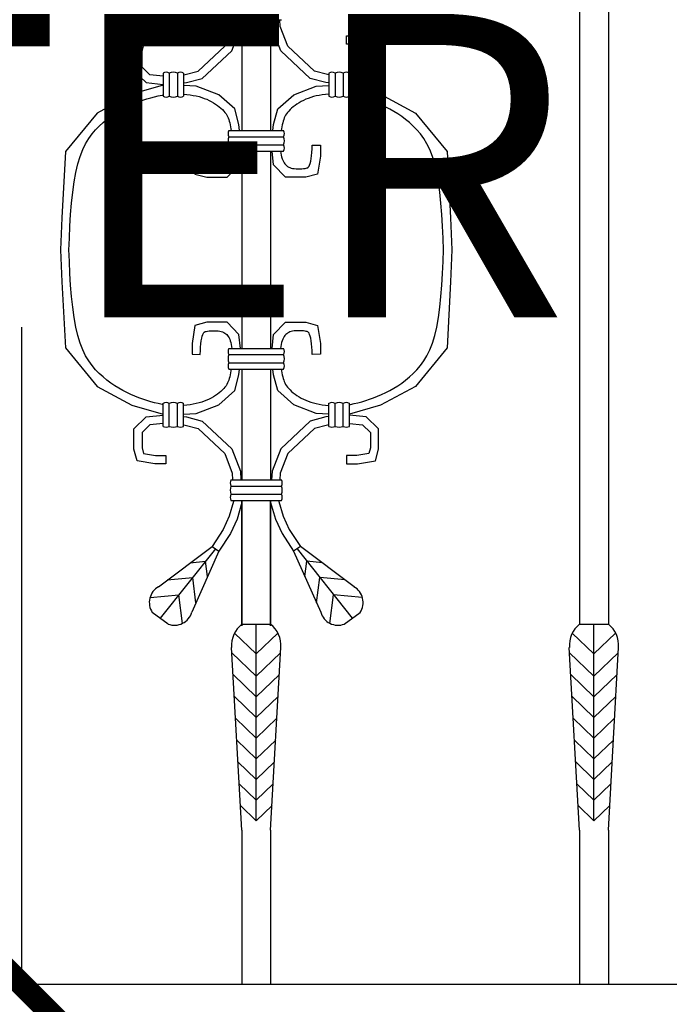
# Model space of a CAD drawing. Units: inches. Extents: x 2278 to 7495, y -71 to 1198.
# Tile 27 of 44: x 5101.34 to 5114.19, y 126.41 to 145.88. Entities that reach past the tile are written whole.
import ezdxf

# ---------------------------------------------------------------- set-up
doc = ezdxf.new("R2010")
doc.units = ezdxf.units.IN
doc.header["$MEASUREMENT"] = 0
doc.layers.add('A-ANNO-DIMS', color=2, linetype='Continuous', lineweight=18)
doc.layers.add('A-ELEV', color=7, linetype='Continuous', lineweight=25)
doc.styles.get("Standard").update_dxf_attribs({"font": 'arial.ttf'})
doc.dimstyles.get("Standard").update_dxf_attribs({"dimtxt": 6, "dimasz": 3, "dimexe": 0.18, "dimexo": 0.0625, "dimgap": 0.09, "dimtad": 0, "dimtih": 1, "dimtoh": 1, "dimdec": 0, "dimzin": 0, "dimdsep": 46, "dimlunit": 3, "dimtxsty": 'Standard', "dimblk": 'ARCHTICK', "dimcen": 0.09, "dimadec": 0, "dimazin": 0, "dimtfac": 1, "dimtdec": 0, "dimtofl": 0, "dimtmove": 0, "dimatfit": 3, "dimfxl": 1, "dimtolj": 1, "dimtzin": 0, "dimarcsym": 0})

# ---------------------------------------------------------------- blocks, each defined once
blk = doc.blocks.new('BALUSTER-ORNATE-A')
for p, q in [((3.37, 19.077), (4.37, 19.077)), ((3.396, 18.942), (3.402, 19.077)), ((3.558, 18.908), (3.565, 19.077)), ((3.585, 19.077), (3.585, 16.887)), ((4.155, 19.077), (4.155, 16.887)), ((4.182, 18.908), (4.175, 19.077)), ((4.344, 18.942), (4.338, 19.077)), ((3.247, 18.557), (3.396, 18.942)), ((3.385, 18.463), (3.558, 18.908)), ((4.355, 18.463), (4.182, 18.908)), ((4.493, 18.557), (4.344, 18.942)), ((1.513, 18.705), (1.449, 18.469)), ((1.866, 18.759), (1.513, 18.705)), ((2.084, 18.759), (1.866, 18.759)), ((2.084, 18.596), (2.084, 18.759)), ((5.656, 18.596), (5.656, 18.759)), ((5.656, 18.759), (5.874, 18.759)), ((5.874, 18.759), (6.227, 18.705)), ((6.227, 18.705), (6.291, 18.469)), ((1.612, 18.447), (1.642, 18.56)), ((1.642, 18.56), (1.879, 18.596)), ((1.879, 18.596), (2.084, 18.596)), ((2.719, 18.062), (3.247, 18.557)), ((5.021, 18.062), (4.493, 18.557)), ((5.861, 18.596), (5.656, 18.596)), ((6.098, 18.56), (5.861, 18.596)), ((6.128, 18.447), (6.098, 18.56)), ((1.449, 18.469), (1.449, 18.069)), ((1.612, 18.138), (1.612, 18.447)), ((2.801, 17.915), (3.385, 18.463)), ((4.939, 17.915), (4.355, 18.463)), ((6.128, 18.138), (6.128, 18.447)), ((6.291, 18.469), (6.291, 18.069)), ((1.767, 17.989), (1.612, 18.138)), ((5.973, 17.989), (6.128, 18.138)), ((1.449, 18.069), (1.694, 17.833)), ((2.026, 17.961), (1.767, 17.989)), ((2.026, 18.021), (2.026, 17.565)), ((2.148, 18.021), (2.148, 17.565)), ((2.311, 18.021), (2.311, 17.565)), ((2.434, 18.021), (2.434, 17.565)), ((2.434, 17.99), (2.462, 17.993)), ((2.462, 17.993), (2.719, 18.062)), ((2.492, 17.833), (2.801, 17.915)), ((5.248, 17.833), (4.939, 17.915)), ((5.278, 17.993), (5.021, 18.062)), ((5.306, 17.99), (5.278, 17.993)), ((5.306, 18.021), (5.306, 17.565)), ((5.429, 18.021), (5.429, 17.565)), ((5.592, 18.021), (5.592, 17.565)), ((5.714, 18.021), (5.714, 17.565)), ((5.714, 17.961), (5.973, 17.989)), ((6.291, 18.069), (6.046, 17.833)), ((2.026, 17.782), (1.412, 17.603)), ((1.694, 17.833), (2.026, 17.797)), ((2.434, 17.826), (2.492, 17.833)), ((2.683, 17.766), (2.434, 17.777)), ((3.128, 17.594), (2.683, 17.766)), ((4.612, 17.594), (5.057, 17.766)), ((5.057, 17.766), (5.306, 17.777)), ((5.306, 17.826), (5.248, 17.833)), ((6.046, 17.833), (5.714, 17.797)), ((5.714, 17.782), (6.328, 17.603)), ((1.412, 17.603), (0.722, 17.231)), ((1.705, 17.51), (1.782, 17.533)), ((1.782, 17.533), (1.858, 17.553)), ((1.858, 17.553), (1.933, 17.571)), ((1.933, 17.571), (2.007, 17.585)), ((2.007, 17.585), (2.026, 17.587)), ((2.434, 17.606), (2.499, 17.6)), ((2.499, 17.6), (2.563, 17.592)), ((2.563, 17.592), (2.624, 17.582)), ((2.624, 17.582), (2.683, 17.57)), ((2.683, 17.57), (2.739, 17.556)), ((2.739, 17.556), (2.792, 17.54)), ((2.792, 17.54), (2.843, 17.522)), ((2.843, 17.522), (2.891, 17.503)), ((3.446, 17.313), (3.128, 17.594)), ((4.294, 17.313), (4.612, 17.594)), ((4.897, 17.522), (4.849, 17.503)), ((4.948, 17.54), (4.897, 17.522)), ((5.001, 17.556), (4.948, 17.54)), ((5.057, 17.57), (5.001, 17.556)), ((5.116, 17.582), (5.057, 17.57)), ((5.177, 17.592), (5.116, 17.582)), ((5.241, 17.6), (5.177, 17.592)), ((5.306, 17.606), (5.241, 17.6)), ((5.733, 17.585), (5.714, 17.587)), ((5.807, 17.571), (5.733, 17.585)), ((5.882, 17.553), (5.807, 17.571)), ((5.958, 17.533), (5.882, 17.553)), ((6.035, 17.51), (5.958, 17.533)), ((6.328, 17.603), (7.018, 17.231)), ((1.23, 17.309), (1.309, 17.35)), ((1.309, 17.35), (1.389, 17.388)), ((1.389, 17.388), (1.469, 17.422)), ((1.469, 17.422), (1.549, 17.454)), ((1.549, 17.454), (1.627, 17.484)), ((1.627, 17.484), (1.705, 17.51)), ((2.891, 17.503), (2.937, 17.482)), ((2.937, 17.482), (2.981, 17.46)), ((2.981, 17.46), (3.024, 17.436)), ((3.024, 17.436), (3.064, 17.41)), ((3.064, 17.41), (3.102, 17.384)), ((3.102, 17.384), (3.138, 17.357)), ((3.138, 17.357), (3.171, 17.329)), ((3.171, 17.329), (3.201, 17.301)), ((4.569, 17.329), (4.539, 17.301)), ((4.602, 17.357), (4.569, 17.329)), ((4.638, 17.384), (4.602, 17.357)), ((4.676, 17.41), (4.638, 17.384)), ((4.716, 17.436), (4.676, 17.41)), ((4.759, 17.46), (4.716, 17.436)), ((4.803, 17.482), (4.759, 17.46)), ((4.849, 17.503), (4.803, 17.482)), ((6.113, 17.484), (6.035, 17.51)), ((6.191, 17.454), (6.113, 17.484)), ((6.271, 17.422), (6.191, 17.454)), ((6.351, 17.388), (6.271, 17.422)), ((6.431, 17.35), (6.351, 17.388)), ((6.51, 17.309), (6.431, 17.35)), ((0.722, 17.231), (0.096, 16.469)), ((0.916, 17.105), (0.993, 17.163)), ((0.993, 17.163), (1.071, 17.216)), ((1.071, 17.216), (1.15, 17.265)), ((1.15, 17.265), (1.23, 17.309)), ((3.201, 17.301), (3.228, 17.272)), ((3.228, 17.272), (3.252, 17.244)), ((3.252, 17.244), (3.272, 17.217)), ((3.272, 17.217), (3.288, 17.19)), ((3.288, 17.19), (3.303, 17.162)), ((3.303, 17.162), (3.316, 17.134)), ((3.316, 17.134), (3.327, 17.104)), ((3.528, 17.004), (3.446, 17.313)), ((4.212, 17.004), (4.294, 17.313)), ((4.424, 17.134), (4.413, 17.104)), ((4.437, 17.162), (4.424, 17.134)), ((4.452, 17.19), (4.437, 17.162)), ((4.468, 17.217), (4.452, 17.19)), ((4.489, 17.244), (4.468, 17.217)), ((4.512, 17.272), (4.489, 17.244)), ((4.539, 17.301), (4.512, 17.272)), ((6.59, 17.265), (6.51, 17.309)), ((6.669, 17.216), (6.59, 17.265)), ((6.747, 17.163), (6.669, 17.216)), ((6.824, 17.105), (6.747, 17.163)), ((7.018, 17.231), (7.644, 16.469)), ((0.692, 16.9), (0.764, 16.975)), ((0.764, 16.975), (0.839, 17.043)), ((0.839, 17.043), (0.916, 17.105)), ((3.327, 17.104), (3.337, 17.072)), ((3.337, 17.072), (3.346, 17.038)), ((3.346, 17.038), (3.354, 17.001)), ((3.354, 17.001), (3.361, 16.962)), ((3.361, 16.962), (3.368, 16.922)), ((3.542, 16.887), (3.528, 17.004)), ((4.198, 16.887), (4.212, 17.004)), ((4.379, 16.962), (4.372, 16.922)), ((4.386, 17.001), (4.379, 16.962)), ((4.394, 17.038), (4.386, 17.001)), ((4.403, 17.072), (4.394, 17.038)), ((4.413, 17.104), (4.403, 17.072)), ((6.901, 17.043), (6.824, 17.105)), ((6.976, 16.975), (6.901, 17.043)), ((7.048, 16.9), (6.976, 16.975)), ((0.557, 16.727), (0.623, 16.819)), ((0.623, 16.819), (0.692, 16.9)), ((3.329, 16.887), (4.411, 16.887)), ((3.329, 16.764), (4.411, 16.764)), ((3.368, 16.922), (3.374, 16.887)), ((4.372, 16.922), (4.366, 16.887)), ((7.117, 16.819), (7.048, 16.9)), ((7.183, 16.727), (7.117, 16.819)), ((0.438, 16.508), (0.495, 16.624)), ((0.495, 16.624), (0.557, 16.727)), ((2.764, 16.599), (2.602, 16.596)), ((2.602, 16.596), (2.602, 16.378)), ((2.766, 16.522), (2.764, 16.599)), ((3.329, 16.601), (4.411, 16.601)), ((4.974, 16.522), (4.976, 16.599)), ((4.976, 16.599), (5.138, 16.596)), ((5.138, 16.596), (5.138, 16.378)), ((7.245, 16.624), (7.183, 16.727)), ((7.302, 16.508), (7.245, 16.624)), ((0.096, 16.469), (0.025, 15.162)), ((0.34, 16.227), (0.386, 16.376)), ((0.386, 16.376), (0.438, 16.508)), ((2.602, 16.378), (2.656, 16.024)), ((2.769, 16.452), (2.766, 16.522)), ((2.775, 16.388), (2.769, 16.452)), ((2.783, 16.331), (2.775, 16.388)), ((3.329, 16.479), (4.411, 16.479)), ((3.368, 16.364), (3.357, 16.329)), ((3.376, 16.401), (3.368, 16.364)), ((3.383, 16.441), (3.376, 16.401)), ((3.388, 16.479), (3.383, 16.441)), ((3.528, 16.206), (3.557, 16.479)), ((3.585, 16.479), (3.585, 12.578)), ((4.155, 16.479), (4.155, 12.578)), ((4.212, 16.206), (4.183, 16.479)), ((4.352, 16.479), (4.357, 16.441)), ((4.357, 16.441), (4.364, 16.401)), ((4.364, 16.401), (4.372, 16.364)), ((4.372, 16.364), (4.383, 16.329)), ((4.957, 16.331), (4.965, 16.388)), ((4.965, 16.388), (4.971, 16.452)), ((4.971, 16.452), (4.974, 16.522)), ((5.138, 16.378), (5.084, 16.024)), ((7.354, 16.376), (7.302, 16.508)), ((7.4, 16.227), (7.354, 16.376)), ((7.644, 16.469), (7.715, 15.162)), ((0.3, 16.057), (0.34, 16.227)), ((2.792, 16.28), (2.783, 16.331)), ((2.803, 16.237), (2.792, 16.28)), ((2.815, 16.203), (2.803, 16.237)), ((2.825, 16.18), (2.815, 16.203)), ((2.834, 16.166), (2.825, 16.18)), ((2.84, 16.159), (2.834, 16.166)), ((2.846, 16.154), (2.84, 16.159)), ((3.228, 16.164), (3.205, 16.154)), ((3.249, 16.176), (3.228, 16.164)), ((3.268, 16.19), (3.249, 16.176)), ((3.286, 16.207), (3.268, 16.19)), ((3.303, 16.225), (3.286, 16.207)), ((3.292, 15.961), (3.528, 16.206)), ((3.318, 16.247), (3.303, 16.225)), ((3.333, 16.271), (3.318, 16.247)), ((3.346, 16.299), (3.333, 16.271)), ((3.357, 16.329), (3.346, 16.299)), ((4.448, 15.961), (4.212, 16.206)), ((4.383, 16.329), (4.394, 16.299)), ((4.394, 16.299), (4.407, 16.271)), ((4.407, 16.271), (4.422, 16.247)), ((4.422, 16.247), (4.437, 16.225)), ((4.437, 16.225), (4.454, 16.207)), ((4.454, 16.207), (4.472, 16.19)), ((4.472, 16.19), (4.491, 16.176)), ((4.491, 16.176), (4.512, 16.164)), ((4.512, 16.164), (4.535, 16.154)), ((4.895, 16.154), (4.9, 16.159)), ((4.9, 16.159), (4.906, 16.166)), ((4.906, 16.166), (4.915, 16.18)), ((4.915, 16.18), (4.925, 16.203)), ((4.925, 16.203), (4.937, 16.237)), ((4.937, 16.237), (4.948, 16.28)), ((4.948, 16.28), (4.957, 16.331)), ((7.44, 16.057), (7.4, 16.227)), ((0.267, 15.87), (0.3, 16.057)), ((2.656, 16.024), (2.892, 15.961)), ((2.852, 16.151), (2.846, 16.154)), ((2.863, 16.146), (2.852, 16.151)), ((2.88, 16.142), (2.863, 16.146)), ((2.905, 16.137), (2.88, 16.142)), ((2.936, 16.134), (2.905, 16.137)), ((2.971, 16.131), (2.936, 16.134)), ((3.008, 16.129), (2.971, 16.131)), ((3.045, 16.129), (3.008, 16.129)), ((3.081, 16.13), (3.045, 16.129)), ((3.117, 16.133), (3.081, 16.13)), ((3.15, 16.138), (3.117, 16.133)), ((3.179, 16.145), (3.15, 16.138)), ((3.205, 16.154), (3.179, 16.145)), ((4.535, 16.154), (4.561, 16.145)), ((4.561, 16.145), (4.59, 16.138)), ((4.59, 16.138), (4.623, 16.133)), ((4.623, 16.133), (4.659, 16.13)), ((4.659, 16.13), (4.695, 16.129)), ((4.695, 16.129), (4.732, 16.129)), ((4.732, 16.129), (4.769, 16.131)), ((4.769, 16.131), (4.804, 16.134)), ((4.804, 16.134), (4.835, 16.137)), ((4.835, 16.137), (4.86, 16.142)), ((5.084, 16.024), (4.848, 15.961)), ((4.86, 16.142), (4.877, 16.146)), ((4.877, 16.146), (4.888, 16.151)), ((4.888, 16.151), (4.895, 16.154)), ((7.473, 15.87), (7.44, 16.057)), ((0.239, 15.667), (0.267, 15.87)), ((2.892, 15.961), (3.292, 15.961)), ((4.848, 15.961), (4.448, 15.961)), ((7.501, 15.667), (7.473, 15.87)), ((0.217, 15.452), (0.239, 15.667)), ((7.523, 15.452), (7.501, 15.667)), ((0.199, 15.227), (0.217, 15.452)), ((7.541, 15.227), (7.523, 15.452)), ((0.185, 14.995), (0.199, 15.227)), ((7.555, 14.995), (7.541, 15.227)), ((0.025, 15.162), (0, 14.529)), ((0.173, 14.759), (0.185, 14.995)), ((7.567, 14.759), (7.555, 14.995)), ((7.715, 15.162), (7.74, 14.529)), ((0.163, 14.522), (0.173, 14.759)), ((7.577, 14.522), (7.567, 14.759)), ((0, 14.529), (0.025, 13.895)), ((0.173, 14.298), (0.163, 14.536)), ((7.567, 14.298), (7.577, 14.536)), ((7.74, 14.529), (7.715, 13.895)), ((0.185, 14.062), (0.173, 14.298)), ((7.555, 14.062), (7.567, 14.298)), ((0.199, 13.831), (0.185, 14.062)), ((7.541, 13.831), (7.555, 14.062)), ((0.025, 13.895), (0.096, 12.589)), ((0.217, 13.606), (0.199, 13.831)), ((7.523, 13.606), (7.541, 13.831)), ((7.715, 13.895), (7.644, 12.589)), ((0.239, 13.391), (0.217, 13.606)), ((7.501, 13.391), (7.523, 13.606)), ((0.267, 13.188), (0.239, 13.391)), ((7.473, 13.188), (7.501, 13.391)), ((0.3, 13), (0.267, 13.188)), ((2.892, 13.097), (2.656, 13.033)), ((3.292, 13.097), (2.892, 13.097)), ((3.528, 12.852), (3.292, 13.097)), ((4.212, 12.852), (4.448, 13.097)), ((4.448, 13.097), (4.848, 13.097)), ((4.848, 13.097), (5.084, 13.033)), ((7.44, 13), (7.473, 13.188)), ((0.34, 12.831), (0.3, 13)), ((2.656, 13.033), (2.602, 12.679)), ((2.803, 12.82), (2.815, 12.854)), ((2.815, 12.854), (2.825, 12.878)), ((2.825, 12.878), (2.834, 12.892)), ((2.834, 12.892), (2.84, 12.899)), ((2.84, 12.899), (2.846, 12.903)), ((2.846, 12.903), (2.852, 12.907)), ((2.852, 12.907), (2.863, 12.911)), ((2.863, 12.911), (2.88, 12.916)), ((2.88, 12.916), (2.905, 12.92)), ((2.905, 12.92), (2.936, 12.924)), ((2.936, 12.924), (2.971, 12.927)), ((2.971, 12.927), (3.008, 12.929)), ((3.008, 12.929), (3.045, 12.929)), ((3.045, 12.929), (3.081, 12.928)), ((3.081, 12.928), (3.117, 12.924)), ((3.117, 12.924), (3.15, 12.919)), ((3.15, 12.919), (3.179, 12.912)), ((3.179, 12.912), (3.205, 12.904)), ((3.205, 12.904), (3.228, 12.893)), ((3.228, 12.893), (3.249, 12.881)), ((3.249, 12.881), (3.268, 12.867)), ((3.268, 12.867), (3.286, 12.851)), ((3.286, 12.851), (3.303, 12.832)), ((3.557, 12.578), (3.528, 12.852)), ((4.183, 12.578), (4.212, 12.852)), ((4.454, 12.851), (4.437, 12.832)), ((4.472, 12.867), (4.454, 12.851)), ((4.491, 12.881), (4.472, 12.867)), ((4.512, 12.893), (4.491, 12.881)), ((4.535, 12.904), (4.512, 12.893)), ((4.561, 12.912), (4.535, 12.904)), ((4.59, 12.919), (4.561, 12.912)), ((4.623, 12.924), (4.59, 12.919)), ((4.659, 12.928), (4.623, 12.924)), ((4.695, 12.929), (4.659, 12.928)), ((4.732, 12.929), (4.695, 12.929)), ((4.769, 12.927), (4.732, 12.929)), ((4.804, 12.924), (4.769, 12.927)), ((4.835, 12.92), (4.804, 12.924)), ((4.86, 12.916), (4.835, 12.92)), ((4.877, 12.911), (4.86, 12.916)), ((4.888, 12.907), (4.877, 12.911)), ((4.895, 12.903), (4.888, 12.907)), ((4.9, 12.899), (4.895, 12.903)), ((4.906, 12.892), (4.9, 12.899)), ((4.915, 12.878), (4.906, 12.892)), ((4.925, 12.854), (4.915, 12.878)), ((4.937, 12.82), (4.925, 12.854)), ((5.084, 13.033), (5.138, 12.679)), ((7.4, 12.831), (7.44, 13)), ((0.386, 12.681), (0.34, 12.831)), ((0.438, 12.549), (0.386, 12.681)), ((2.602, 12.679), (2.602, 12.462)), ((2.769, 12.605), (2.775, 12.669)), ((2.775, 12.669), (2.783, 12.727)), ((2.783, 12.727), (2.792, 12.778)), ((2.792, 12.778), (2.803, 12.82)), ((3.303, 12.832), (3.318, 12.811)), ((3.318, 12.811), (3.333, 12.786)), ((3.333, 12.786), (3.346, 12.759)), ((3.346, 12.759), (3.357, 12.728)), ((3.357, 12.728), (3.368, 12.694)), ((3.368, 12.694), (3.376, 12.656)), ((3.376, 12.656), (3.383, 12.616)), ((4.364, 12.656), (4.357, 12.616)), ((4.372, 12.694), (4.364, 12.656)), ((4.383, 12.728), (4.372, 12.694)), ((4.394, 12.759), (4.383, 12.728)), ((4.407, 12.786), (4.394, 12.759)), ((4.422, 12.811), (4.407, 12.786)), ((4.437, 12.832), (4.422, 12.811)), ((4.948, 12.778), (4.937, 12.82)), ((4.957, 12.727), (4.948, 12.778)), ((4.965, 12.669), (4.957, 12.727)), ((4.971, 12.605), (4.965, 12.669)), ((5.138, 12.679), (5.138, 12.462)), ((7.302, 12.549), (7.354, 12.681)), ((7.354, 12.681), (7.4, 12.831)), ((0.096, 12.589), (0.722, 11.827)), ((0.495, 12.433), (0.438, 12.549)), ((2.602, 12.462), (2.764, 12.459)), ((2.764, 12.459), (2.766, 12.536)), ((2.766, 12.536), (2.769, 12.605)), ((3.329, 12.578), (4.411, 12.578)), ((3.383, 12.616), (3.388, 12.578)), ((4.357, 12.616), (4.352, 12.578)), ((4.974, 12.536), (4.971, 12.605)), ((4.976, 12.459), (4.974, 12.536)), ((5.138, 12.462), (4.976, 12.459)), ((7.644, 12.589), (7.018, 11.827)), ((7.245, 12.433), (7.302, 12.549)), ((0.557, 12.33), (0.495, 12.433)), ((0.623, 12.239), (0.557, 12.33)), ((3.329, 12.456), (4.411, 12.456)), ((3.329, 12.293), (4.411, 12.293)), ((7.117, 12.239), (7.183, 12.33)), ((7.183, 12.33), (7.245, 12.433)), ((0.692, 12.157), (0.623, 12.239)), ((0.764, 12.083), (0.692, 12.157)), ((0.839, 12.015), (0.764, 12.083)), ((3.329, 12.171), (4.411, 12.171)), ((3.361, 12.095), (3.354, 12.056)), ((3.368, 12.136), (3.361, 12.095)), ((3.374, 12.171), (3.368, 12.136)), ((3.528, 12.053), (3.542, 12.171)), ((3.585, 12.171), (3.585, 9.98)), ((4.155, 12.171), (4.155, 9.98)), ((4.212, 12.053), (4.198, 12.171)), ((4.366, 12.171), (4.372, 12.136)), ((4.372, 12.136), (4.379, 12.095)), ((4.379, 12.095), (4.386, 12.056)), ((6.901, 12.015), (6.976, 12.083)), ((6.976, 12.083), (7.048, 12.157)), ((7.048, 12.157), (7.117, 12.239)), ((0.916, 11.952), (0.839, 12.015)), ((0.993, 11.894), (0.916, 11.952)), ((1.071, 11.841), (0.993, 11.894)), ((3.303, 11.895), (3.288, 11.868)), ((3.316, 11.924), (3.303, 11.895)), ((3.327, 11.954), (3.316, 11.924)), ((3.337, 11.986), (3.327, 11.954)), ((3.346, 12.02), (3.337, 11.986)), ((3.354, 12.056), (3.346, 12.02)), ((3.446, 11.745), (3.528, 12.053)), ((4.294, 11.745), (4.212, 12.053)), ((4.386, 12.056), (4.394, 12.02)), ((4.394, 12.02), (4.403, 11.986)), ((4.403, 11.986), (4.413, 11.954)), ((4.413, 11.954), (4.424, 11.924)), ((4.424, 11.924), (4.437, 11.895)), ((4.437, 11.895), (4.452, 11.868)), ((6.669, 11.841), (6.747, 11.894)), ((6.747, 11.894), (6.824, 11.952)), ((6.824, 11.952), (6.901, 12.015)), ((0.722, 11.827), (1.412, 11.455)), ((1.15, 11.793), (1.071, 11.841)), ((1.23, 11.748), (1.15, 11.793)), ((1.309, 11.708), (1.23, 11.748)), ((1.389, 11.67), (1.309, 11.708)), ((3.138, 11.701), (3.102, 11.673)), ((3.128, 11.464), (3.446, 11.745)), ((3.171, 11.729), (3.138, 11.701)), ((3.201, 11.757), (3.171, 11.729)), ((3.228, 11.785), (3.201, 11.757)), ((3.252, 11.813), (3.228, 11.785)), ((3.272, 11.841), (3.252, 11.813)), ((3.288, 11.868), (3.272, 11.841)), ((4.612, 11.464), (4.294, 11.745)), ((4.452, 11.868), (4.468, 11.841)), ((4.468, 11.841), (4.489, 11.813)), ((4.489, 11.813), (4.512, 11.785)), ((4.512, 11.785), (4.539, 11.757)), ((4.539, 11.757), (4.569, 11.729)), ((4.569, 11.729), (4.602, 11.701)), ((4.602, 11.701), (4.638, 11.673)), ((7.018, 11.827), (6.328, 11.455)), ((6.351, 11.67), (6.431, 11.708)), ((6.431, 11.708), (6.51, 11.748)), ((6.51, 11.748), (6.59, 11.793)), ((6.59, 11.793), (6.669, 11.841)), ((1.469, 11.635), (1.389, 11.67)), ((1.549, 11.603), (1.469, 11.635)), ((1.627, 11.574), (1.549, 11.603)), ((1.705, 11.548), (1.627, 11.574)), ((1.782, 11.524), (1.705, 11.548)), ((1.858, 11.504), (1.782, 11.524)), ((1.933, 11.487), (1.858, 11.504)), ((2.007, 11.473), (1.933, 11.487)), ((2.026, 11.037), (2.026, 11.493)), ((2.148, 11.037), (2.148, 11.493)), ((2.311, 11.037), (2.311, 11.493)), ((2.434, 11.037), (2.434, 11.493)), ((2.683, 11.488), (2.624, 11.476)), ((2.739, 11.502), (2.683, 11.488)), ((2.792, 11.518), (2.739, 11.502)), ((2.843, 11.535), (2.792, 11.518)), ((2.891, 11.555), (2.843, 11.535)), ((2.937, 11.576), (2.891, 11.555)), ((2.981, 11.598), (2.937, 11.576)), ((3.024, 11.622), (2.981, 11.598)), ((3.064, 11.647), (3.024, 11.622)), ((3.102, 11.673), (3.064, 11.647)), ((4.638, 11.673), (4.676, 11.647)), ((4.676, 11.647), (4.716, 11.622)), ((4.716, 11.622), (4.759, 11.598)), ((4.759, 11.598), (4.803, 11.576)), ((4.803, 11.576), (4.849, 11.555)), ((4.849, 11.555), (4.897, 11.535)), ((4.897, 11.535), (4.948, 11.518)), ((4.948, 11.518), (5.001, 11.502)), ((5.001, 11.502), (5.057, 11.488)), ((5.057, 11.488), (5.116, 11.476)), ((5.306, 11.037), (5.306, 11.493)), ((5.429, 11.037), (5.429, 11.493)), ((5.592, 11.037), (5.592, 11.493)), ((5.714, 11.037), (5.714, 11.493)), ((5.733, 11.473), (5.807, 11.487)), ((5.807, 11.487), (5.882, 11.504)), ((5.882, 11.504), (5.958, 11.524)), ((5.958, 11.524), (6.035, 11.548)), ((6.035, 11.548), (6.113, 11.574)), ((6.113, 11.574), (6.191, 11.603)), ((6.191, 11.603), (6.271, 11.635)), ((6.271, 11.635), (6.351, 11.67)), ((1.412, 11.455), (2.026, 11.276)), ((2.026, 11.47), (2.007, 11.473)), ((2.499, 11.457), (2.434, 11.451)), ((2.434, 11.28), (2.683, 11.291)), ((2.563, 11.465), (2.499, 11.457)), ((2.624, 11.476), (2.563, 11.465)), ((2.683, 11.291), (3.128, 11.464)), ((5.057, 11.291), (4.612, 11.464)), ((5.306, 11.28), (5.057, 11.291)), ((5.116, 11.476), (5.177, 11.465)), ((5.177, 11.465), (5.241, 11.457)), ((5.241, 11.457), (5.306, 11.451)), ((5.714, 11.47), (5.733, 11.473)), ((6.328, 11.455), (5.714, 11.276)), ((1.449, 10.988), (1.694, 11.225)), ((1.694, 11.225), (2.026, 11.261)), ((2.026, 11.097), (1.767, 11.069)), ((2.434, 11.232), (2.492, 11.225)), ((2.492, 11.225), (2.801, 11.143)), ((2.801, 11.143), (3.385, 10.594)), ((4.939, 11.143), (4.355, 10.594)), ((5.248, 11.225), (4.939, 11.143)), ((5.306, 11.232), (5.248, 11.225)), ((6.046, 11.225), (5.714, 11.261)), ((5.714, 11.097), (5.973, 11.069)), ((6.291, 10.988), (6.046, 11.225)), ((1.449, 10.589), (1.449, 10.988)), ((1.767, 11.069), (1.612, 10.919)), ((1.612, 10.919), (1.612, 10.611)), ((2.434, 11.067), (2.462, 11.064)), ((2.462, 11.064), (2.719, 10.996)), ((2.719, 10.996), (3.247, 10.501)), ((5.021, 10.996), (4.493, 10.501)), ((5.278, 11.064), (5.021, 10.996)), ((5.306, 11.067), (5.278, 11.064)), ((5.973, 11.069), (6.128, 10.919)), ((6.128, 10.919), (6.128, 10.611)), ((6.291, 10.589), (6.291, 10.988)), ((1.513, 10.353), (1.449, 10.589)), ((1.612, 10.611), (1.642, 10.498)), ((3.385, 10.594), (3.558, 10.149)), ((4.355, 10.594), (4.182, 10.149)), ((6.128, 10.611), (6.098, 10.498)), ((6.227, 10.353), (6.291, 10.589)), ((1.866, 10.298), (1.513, 10.353)), ((1.642, 10.498), (1.879, 10.461)), ((1.879, 10.461), (2.084, 10.461)), ((2.084, 10.461), (2.084, 10.298)), ((3.247, 10.501), (3.396, 10.115)), ((4.493, 10.501), (4.344, 10.115)), ((5.861, 10.461), (5.656, 10.461)), ((5.656, 10.461), (5.656, 10.298)), ((6.098, 10.498), (5.861, 10.461)), ((5.874, 10.298), (6.227, 10.353)), ((2.084, 10.298), (1.866, 10.298)), ((3.558, 10.149), (3.565, 9.98)), ((4.182, 10.149), (4.175, 9.98)), ((5.656, 10.298), (5.874, 10.298)), ((3.37, 9.98), (4.37, 9.98)), ((3.396, 10.115), (3.402, 9.98)), ((4.344, 10.115), (4.338, 9.98)), ((3.37, 9.858), (4.37, 9.858)), ((3.421, 9.552), (3.337, 9.262)), ((3.37, 9.695), (4.37, 9.695)), ((3.37, 9.573), (4.37, 9.573)), ((3.42, 9.573), (3.421, 9.552)), ((3.583, 9.573), (3.585, 9.532)), ((3.585, 9.573), (3.585, 7.095)), ((3.585, 7.095), (3.585, 9.573)), ((4.155, 9.573), (4.155, 7.095)), ((4.155, 7.095), (4.155, 9.573)), ((4.157, 9.573), (4.155, 9.532)), ((4.32, 9.573), (4.319, 9.552)), ((4.319, 9.552), (4.403, 9.262)), ((3.585, 9.532), (3.49, 9.205)), ((4.155, 9.532), (4.25, 9.205)), ((3.337, 9.262), (3.217, 9.001)), ((3.49, 9.205), (3.36, 8.922)), ((4.25, 9.205), (4.38, 8.922)), ((4.403, 9.262), (4.523, 9.001)), ((3.217, 9.001), (2.995, 8.66)), ((4.523, 9.001), (4.745, 8.66)), ((3.36, 8.922), (3.131, 8.571)), ((4.38, 8.922), (4.609, 8.571)), ((1.936, 7.866), (2.995, 8.66)), ((3.063, 8.615), (1.97, 7.244)), ((3.131, 8.571), (2.594, 7.362)), ((2.995, 8.66), (3.131, 8.571)), ((4.745, 8.66), (4.609, 8.571)), ((4.609, 8.571), (5.146, 7.362)), ((4.677, 8.615), (5.77, 7.244)), ((5.804, 7.866), (4.745, 8.66)), ((2.562, 8.34), (2.868, 8.37)), ((2.907, 8.066), (2.868, 8.37)), ((4.833, 8.066), (4.872, 8.37)), ((5.178, 8.34), (4.872, 8.37)), ((2.111, 8.002), (2.613, 8.051)), ((2.678, 7.551), (2.613, 8.051)), ((5.062, 7.551), (5.127, 8.051)), ((5.629, 8.002), (5.127, 8.051)), ((1.774, 7.651), (2.339, 7.706)), ((2.412, 7.143), (2.339, 7.706)), ((5.328, 7.143), (5.401, 7.706)), ((5.966, 7.651), (5.401, 7.706)), ((2.128, 7.128), (1.813, 7.359)), ((5.612, 7.128), (5.927, 7.359)), ((3.585, 7.128), (4.155, 7.128)), ((3.87, 3.24), (3.87, 7.128)), ((3.442, 6.952), (3.87, 6.538)), ((4.299, 6.952), (3.87, 6.538)), ((3.585, 3.055), (3.383, 6.664)), ((4.155, 3.055), (4.357, 6.664)), ((3.388, 6.562), (3.87, 6.097)), ((4.352, 6.562), (3.87, 6.097)), ((3.413, 6.131), (3.87, 5.689)), ((4.327, 6.131), (3.87, 5.689)), ((3.437, 5.699), (3.87, 5.28)), ((4.303, 5.699), (3.87, 5.28)), ((3.461, 5.268), (3.87, 4.872)), ((4.279, 5.268), (3.87, 4.872)), ((3.485, 4.836), (3.87, 4.464)), ((4.255, 4.836), (3.87, 4.464)), ((3.509, 4.405), (3.87, 4.056)), ((4.231, 4.405), (3.87, 4.056)), ((3.533, 3.973), (3.87, 3.648)), ((4.207, 3.973), (3.87, 3.648)), ((3.558, 3.542), (3.87, 3.24)), ((4.182, 3.542), (3.87, 3.24)), ((3.585, 3.055), (3.585, 0)), ((4.155, 3.055), (4.155, 0))]:
    blk.add_line(p, q)
for centre, radius, start, end in [((2.087, 17.916), 0.121, 59.7768, 120.2232), ((2.23, 17.828), 0.209, 67.1017, 112.8983), ((2.373, 17.916), 0.121, 59.7768, 120.2232), ((5.368, 17.916), 0.121, 59.7768, 120.2232), ((5.51, 17.828), 0.209, 67.1017, 112.8983), ((5.653, 17.916), 0.121, 59.7768, 120.2232), ((2.087, 17.67), 0.121, 239.7768, 300.2232), ((2.23, 17.758), 0.209, 247.1017, 292.8983), ((2.373, 17.67), 0.121, 239.7768, 300.2232), ((5.368, 17.67), 0.121, 239.7768, 300.2232), ((5.51, 17.758), 0.209, 247.1017, 292.8983), ((5.653, 17.67), 0.121, 239.7768, 300.2232), ((3.434, 16.825), 0.121, 149.7768, 210.2232), ((3.522, 16.683), 0.209, 157.1017, 202.8983), ((4.306, 16.825), 0.121, 329.7768, 30.2232), ((4.218, 16.683), 0.209, 337.1017, 22.8983), ((3.434, 16.54), 0.121, 149.7768, 210.2232), ((4.306, 16.54), 0.121, 329.7768, 30.2232), ((3.434, 12.517), 0.121, 149.7768, 210.2232), ((4.306, 12.517), 0.121, 329.7768, 30.2232), ((3.522, 12.375), 0.209, 157.1017, 202.8983), ((3.434, 12.232), 0.121, 149.7768, 210.2232), ((4.218, 12.375), 0.209, 337.1017, 22.8983), ((4.306, 12.232), 0.121, 329.7768, 30.2232), ((2.087, 11.388), 0.121, 59.7768, 120.2232), ((2.23, 11.3), 0.209, 67.1017, 112.8983), ((2.373, 11.388), 0.121, 59.7768, 120.2232), ((5.368, 11.388), 0.121, 59.7768, 120.2232), ((5.51, 11.3), 0.209, 67.1017, 112.8983), ((5.653, 11.388), 0.121, 59.7768, 120.2232), ((2.087, 11.142), 0.121, 239.7768, 300.2232), ((2.23, 11.23), 0.209, 247.1017, 292.8983), ((2.373, 11.142), 0.121, 239.7768, 300.2232), ((5.368, 11.142), 0.121, 239.7768, 300.2232), ((5.51, 11.23), 0.209, 247.1017, 292.8983), ((5.653, 11.142), 0.121, 239.7768, 300.2232), ((3.475, 9.919), 0.121, 149.7768, 210.2232), ((4.265, 9.919), 0.121, 329.7768, 30.2232), ((3.563, 9.776), 0.209, 157.1017, 202.8983), ((4.177, 9.776), 0.209, 337.1017, 22.8983), ((3.475, 9.634), 0.121, 149.7768, 210.2232), ((4.265, 9.634), 0.121, 329.7768, 30.2232), ((2.111, 7.555), 0.356, 119.3212, 213.425), ((5.629, 7.555), 0.356, 326.575, 60.6788), ((2.253, 7.462), 0.356, 249.4937, 343.5975), ((5.487, 7.462), 0.356, 196.4025, 290.5063), ((3.929, 6.703), 0.547, 128.9283, 183.9822), ((3.811, 6.703), 0.547, 356.0178, 51.0717)]:
    blk.add_arc(centre, radius, start, end)
blk = doc.blocks.new('RAIL-BAR-C')
for p, q in [((0.203, 21.929), (0.203, 7.128)), ((0.773, 21.929), (0.773, 7.128)), ((0.203, 7.128), (0.773, 7.128)), ((0.488, 3.24), (0.488, 7.128)), ((0.059, 6.952), (0.488, 6.538)), ((0.916, 6.952), (0.488, 6.538)), ((0.203, 3.055), (0, 6.664)), ((0.773, 3.055), (0.975, 6.664)), ((0.006, 6.562), (0.488, 6.097)), ((0.969, 6.562), (0.488, 6.097)), ((0.03, 6.131), (0.488, 5.689)), ((0.945, 6.131), (0.488, 5.689)), ((0.054, 5.699), (0.488, 5.28)), ((0.921, 5.699), (0.488, 5.28)), ((0.079, 5.268), (0.488, 4.872)), ((0.897, 5.268), (0.488, 4.872)), ((0.103, 4.836), (0.488, 4.464)), ((0.873, 4.836), (0.488, 4.464)), ((0.127, 4.405), (0.488, 4.056)), ((0.848, 4.405), (0.488, 4.056)), ((0.151, 3.973), (0.488, 3.648)), ((0.824, 3.973), (0.488, 3.648)), ((0.175, 3.542), (0.488, 3.24)), ((0.8, 3.542), (0.488, 3.24)), ((0.203, 3.055), (0.203, 0)), ((0.773, 3.055), (0.773, 0))]:
    blk.add_line(p, q)
for centre, start, end in [((0.547, 6.703), 128.9283, 183.9822), ((0.429, 6.703), 356.0178, 51.0717)]:
    blk.add_arc(centre, 0.547, start, end)
blk = doc.blocks.new('_ArchTick')
at = {"color": 0, "linetype": 'ByBlock', "const_width": 0.15}
blk.add_lwpolyline([(-0.5, -0.5), (0.5, 0.5)], dxfattribs=at)
blk = doc.blocks.new('*D59')
at = {"layer": 'A-ANNO-DIMS', "color": 0, "lineweight": -2, "transparency": 16777216}
for p, q in [((5096.589, 159.183), (5101.564, 159.183)), ((5101.384, 159.183), (5101.384, 146.185)), ((5101.384, 126.799), (5101.384, 139.796)), ((5096.589, 126.799), (5101.564, 126.799))]:
    blk.add_line(p, q, dxfattribs=at)
at = {"layer": 'Defpoints', "color": 0, "transparency": 16777216}
for p in [(5096.527, 159.183), (5101.384, 159.183), (5096.527, 126.799)]:
    blk.add_point(p, dxfattribs=at)
at = {"layer": 'A-ANNO-DIMS', "color": 0, "lineweight": -2, "transparency": 16777216, "xscale": 3, "yscale": 3, "zscale": 3}
for p, rotation in [((5101.384, 159.183), 90), ((5101.384, 126.799), 270)]:
    blk.add_blockref('_ArchTick', p, dxfattribs=dict(at, rotation=rotation))
at = {"layer": 'A-ANNO-DIMS', "color": 0, "transparency": 16777216, "insert": (5101.384, 142.991), "char_height": 6, "attachment_point": 5}
blk.add_mtext('\\A1;ORNATE BALUSTER 2\'-8 1/2" TYP.', dxfattribs=at)
blk = doc.blocks.new('*D60')
at = {"layer": 'A-ANNO-DIMS', "color": 0, "lineweight": -2, "transparency": 16777216}
for p, q in [((5088.787, 126.736), (5088.787, 121.761)), ((5096.527, 126.736), (5096.527, 121.761)), ((5088.787, 121.941), (5096.527, 121.941)), ((5096.527, 121.941), (5099.527, 121.941))]:
    blk.add_line(p, q, dxfattribs=at)
at = {"layer": 'Defpoints', "color": 0, "transparency": 16777216}
for p in [(5088.787, 126.799), (5096.527, 126.799), (5096.527, 121.941)]:
    blk.add_point(p, dxfattribs=at)
at = {"layer": 'A-ANNO-DIMS', "color": 0, "lineweight": -2, "transparency": 16777216, "xscale": 3, "yscale": 3, "zscale": 3, "rotation": 180}
blk.add_blockref('_ArchTick', (5088.787, 121.941), dxfattribs=at)
at = {"layer": 'A-ANNO-DIMS', "color": 0, "lineweight": -2, "transparency": 16777216, "xscale": 3, "yscale": 3, "zscale": 3}
blk.add_blockref('_ArchTick', (5096.527, 121.941), dxfattribs=at)
at = {"layer": 'A-ANNO-DIMS', "color": 0, "transparency": 16777216, "insert": (5124.894, 121.941), "char_height": 6, "attachment_point": 5}
blk.add_mtext('\\A1;0\'-7 1/2" TYP.', dxfattribs=at)
blk = doc.blocks.new('*D123')
at = {"layer": 'A-ANNO-DIMS', "color": 0, "lineweight": -2, "transparency": 16777216}
for p, q in [((4736.95, 340.157), (4736.95, -23.427)), ((5145.676, -1.81), (5145.676, -23.427)), ((4736.95, -23.247), (4923.929, -23.247)), ((5145.676, -23.247), (4958.697, -23.247))]:
    blk.add_line(p, q, dxfattribs=at)
at = {"layer": 'Defpoints', "color": 0, "transparency": 16777216}
for p in [(4736.95, 340.219), (5145.676, -1.747), (5145.676, -23.247)]:
    blk.add_point(p, dxfattribs=at)
at = {"layer": 'A-ANNO-DIMS', "color": 0, "lineweight": -2, "transparency": 16777216, "xscale": 3, "yscale": 3, "zscale": 3, "rotation": 180}
blk.add_blockref('_ArchTick', (4736.95, -23.247), dxfattribs=at)
at = {"layer": 'A-ANNO-DIMS', "color": 0, "lineweight": -2, "transparency": 16777216, "xscale": 3, "yscale": 3, "zscale": 3}
blk.add_blockref('_ArchTick', (5145.676, -23.247), dxfattribs=at)
at = {"layer": 'A-ANNO-DIMS', "color": 0, "transparency": 16777216, "insert": (4941.313, -23.247), "char_height": 6, "attachment_point": 5}
blk.add_mtext('\\A1;34\'-0 1/2"', dxfattribs=at)
blk = doc.blocks.new('*D131')
at = {"layer": 'A-ANNO-DIMS', "color": 0, "lineweight": -2, "transparency": 16777216}
for p, q in [((5096.176, 99.315), (5096.176, 361.899)), ((5145.676, 118.315), (5145.676, 361.899)), ((5096.176, 361.719), (5105.75, 361.719)), ((5145.676, 361.719), (5136.102, 361.719))]:
    blk.add_line(p, q, dxfattribs=at)
at = {"layer": 'Defpoints', "color": 0, "transparency": 16777216}
for p in [(5145.676, 361.719), (5145.676, 118.253), (5096.176, 99.253)]:
    blk.add_point(p, dxfattribs=at)
at = {"layer": 'A-ANNO-DIMS', "color": 0, "lineweight": -2, "transparency": 16777216, "xscale": 3, "yscale": 3, "zscale": 3, "rotation": 180}
blk.add_blockref('_ArchTick', (5096.176, 361.719), dxfattribs=at)
at = {"layer": 'A-ANNO-DIMS', "color": 0, "lineweight": -2, "transparency": 16777216, "xscale": 3, "yscale": 3, "zscale": 3}
blk.add_blockref('_ArchTick', (5145.676, 361.719), dxfattribs=at)
at = {"layer": 'A-ANNO-DIMS', "color": 0, "transparency": 16777216, "insert": (5120.926, 361.719), "char_height": 6, "attachment_point": 5}
blk.add_mtext('\\A1;4\'-1 1/2"', dxfattribs=at)
blk = doc.blocks.new('*D139')
at = {"layer": 'A-ANNO-DIMS', "color": 0, "lineweight": -2, "transparency": 16777216}
for p, q in [((5092.239, 160.253), (5167.754, 160.253)), ((5167.574, 160.253), (5167.574, 142.408)), ((5167.574, 118.253), (5167.574, 136.097)), ((5145.739, 118.253), (5167.754, 118.253))]:
    blk.add_line(p, q, dxfattribs=at)
at = {"layer": 'Defpoints', "color": 0, "transparency": 16777216}
for p in [(5092.176, 160.253), (5167.574, 160.253), (5145.676, 118.253)]:
    blk.add_point(p, dxfattribs=at)
at = {"layer": 'A-ANNO-DIMS', "color": 0, "lineweight": -2, "transparency": 16777216, "xscale": 3, "yscale": 3, "zscale": 3}
for p, rotation in [((5167.574, 160.253), 90), ((5167.574, 118.253), 270)]:
    blk.add_blockref('_ArchTick', p, dxfattribs=dict(at, rotation=rotation))
at = {"layer": 'A-ANNO-DIMS', "color": 0, "transparency": 16777216, "insert": (5167.574, 139.253), "char_height": 6, "attachment_point": 5}
blk.add_mtext('\\A1;3\'-6"', dxfattribs=at)

msp = doc.modelspace()

# ---------------------------------------------------------------- linework, layer by layer
at = {"layer": 'A-ELEV'}
msp.add_line((5145.676, 126.799), (5066.016, 126.799), dxfattribs=at)

# ---------------------------------------------------------------- block references
for name, p in [('BALUSTER-ORNATE-A', (5102.148, 126.799)), ('RAIL-BAR-C', (5112.211, 126.799))]:
    msp.add_blockref(name, p, dxfattribs=at)

# ---------------------------------------------------------------- dimensions: what is measured, and where the dimension line sits
at = {"layer": 'A-ANNO-DIMS'}
for base, p1, p2, picture, middle in [((5145.676, 361.719), (5096.176, 99.253), (5145.676, 118.253), '*D131', (5120.926, 361.719)), ((5145.676, -23.247), (4736.95, 340.219), (5145.676, -1.747), '*D123', (4941.313, -23.247))]:
    dim = msp.add_linear_dim(base=base, p1=p1, p2=p2, dimstyle='Standard', override={"dimdec": 1, "dimlfac": 1, "dimrnd": 0, "dimzin": 1, "dimdsep": 46, "dimlunit": 4, "dimfrac": 2}, dxfattribs=at)
    dim.commit()
    dim.dimension.update_dxf_attribs({"geometry": picture, "text_midpoint": middle})
dim = msp.add_linear_dim(base=(5101.384, 159.183), p1=(5096.527, 126.799), p2=(5096.527, 159.183), angle=90, text='ORNATE BALUSTER <> TYP.', dimstyle='Standard', override={"dimdec": 1, "dimrnd": 0, "dimzin": 1, "dimlunit": 4, "dimfrac": 2}, dxfattribs=at)
dim.commit()
dim.dimension.update_dxf_attribs({"geometry": '*D59', "text_midpoint": (5101.384, 142.991)})
dim = msp.add_linear_dim(base=(5167.574, 160.253), p1=(5145.676, 118.253), p2=(5092.176, 160.253), angle=90, dimstyle='Standard', override={"dimdec": 1, "dimlfac": 1, "dimrnd": 0, "dimzin": 1, "dimdsep": 46, "dimlunit": 4, "dimfrac": 2}, dxfattribs=at)
dim.commit()
dim.dimension.update_dxf_attribs({"geometry": '*D139', "text_midpoint": (5167.574, 139.253)})
dim = msp.add_linear_dim(base=(5096.527, 121.941), p1=(5088.787, 126.799), p2=(5096.527, 126.799), text='<> TYP.', dimstyle='Standard', override={"dimdec": 1, "dimrnd": 0, "dimzin": 1, "dimlunit": 4, "dimfrac": 2}, dxfattribs=at)
dim.commit()
dim.dimension.update_dxf_attribs({"geometry": '*D60', "text_midpoint": (5124.894, 121.941)})

doc.saveas('drawing.dxf')
